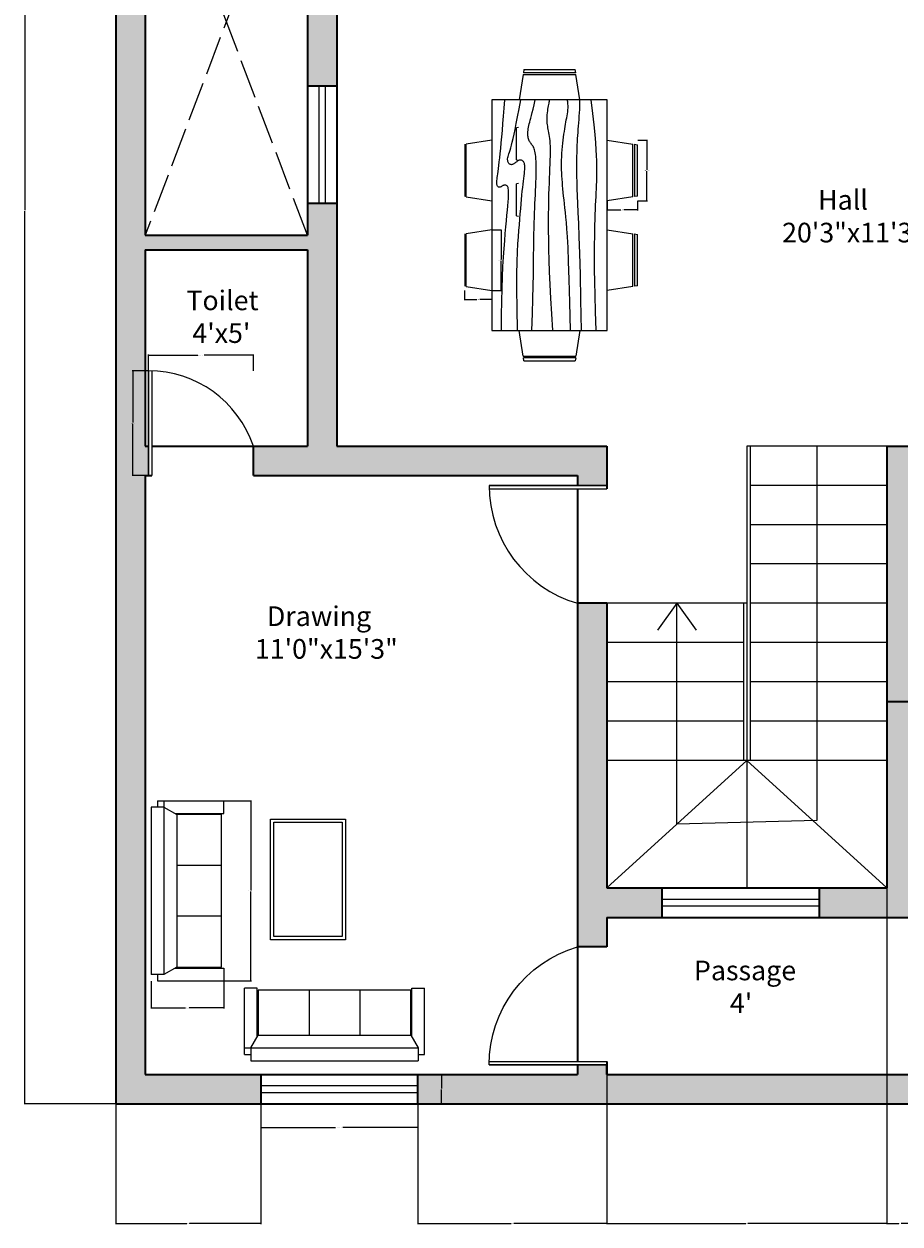
# Model space of a CAD drawing. Units: inches. Extents: x 1752 to 2227, y 6273 to 6884.
# Tile 1 of 6: x 1752 to 2020, y 6273 to 6640. Entities that reach past the tile are written whole.
import ezdxf

# ---------------------------------------------------------------- set-up
doc = ezdxf.new("R2010")
doc.units = ezdxf.units.IN
doc.header["$MEASUREMENT"] = 0
doc.linetypes.add('ACAD_ISO02W100', pattern=[15, 12, -3])
for name, color, linetype, lineweight in [('A-ANNO-DIMS', 2, 'Continuous', 18), ('A-AREA-IDEN', 7, 'Continuous', 18), ('A-DOOR', 3, 'Continuous', 20), ('A-FLOR-STRS', 7, 'Continuous', 20), ('A-FLOR-VOID', 8, 'ACAD_ISO02W100', 13), ('A-FURN', 8, 'Continuous', 18), ('A-GLAZ', 4, 'Continuous', 18), ('A-WALL', 7, 'Continuous', 35)]:
    doc.layers.add(name, color=color, linetype=linetype, lineweight=lineweight)
doc.layers.add('A-WALL-PATT', color=32, linetype='Continuous', lineweight=13, true_color=0xcd6928)
doc.styles.get("Standard").update_dxf_attribs({"font": 'arial.ttf'})
doc.dimstyles.get("Standard").update_dxf_attribs({"dimtxt": 0.18, "dimasz": 0.18, "dimexe": 0.18, "dimexo": 0.0625, "dimgap": 0.09, "dimtad": 0, "dimtih": 1, "dimtoh": 1, "dimdec": 4, "dimzin": 0, "dimdsep": 46, "dimtxsty": 'Standard', "dimcen": 0.09, "dimadec": 0, "dimazin": 0, "dimtfac": 1, "dimtdec": 4, "dimtofl": 0, "dimtmove": 0, "dimatfit": 3, "dimfxl": 1, "dimtolj": 1, "dimtzin": 0, "dimarcsym": 0})

# ---------------------------------------------------------------- blocks, each defined once
blk = doc.blocks.new('SOFA-TWO-SEAT')
for p, q in [((1.96, 55.04), (22.23, 55.04)), ((1.96, 55.04), (1.96, 53.08)), ((3.92, 55.04), (3.92, 1.96)), ((22.23, 51.12), (22.23, 55.04)), ((0, 53.08), (0, 1.96)), ((3.92, 53.08), (0, 53.08)), ((3.92, 53.08), (7.85, 50.88)), ((7.54, 51.12), (22.23, 51.12)), ((21.58, 50.87), (7.85, 50.87)), ((21.58, 35.3), (7.85, 35.3)), ((21.58, 19.74), (7.85, 19.74)), ((7.85, 4.17), (3.92, 1.96)), ((7.29, 3.92), (22.23, 3.92)), ((22.23, 3.92), (22.23, 0)), ((3.92, 1.96), (0, 1.96)), ((1.96, 1.96), (1.96, 0)), ((1.96, 0), (22.23, 0))]:
    blk.add_line(p, q)
blk.add_lwpolyline([(7.85, 50.88), (7.85, 4.17), (21.58, 4.17), (21.58, 50.87)])
blk = doc.blocks.new('CHAIR-DINING')
for p, q in [((0, 18.56), (7.83, 17.34)), ((7.83, 1.23), (7.83, 17.34)), ((8.32, 17.26), (8.32, 1.3)), ((8.32, 17.26), (9.3, 17.11)), ((9.3, 1.45), (9.3, 17.11)), ((7.83, 1.22), (0, 0)), ((9.3, 1.45), (8.32, 1.3))]:
    blk.add_line(p, q)
blk = doc.blocks.new('CHAIR-DINING-SIDE')
for p, q in [((8.32, 18.56), (0.49, 17.34)), ((0, 17.26), (0, 1.3)), ((0.49, 1.23), (0.49, 17.34)), ((0.49, 1.22), (8.32, 0))]:
    blk.add_line(p, q)
blk = doc.blocks.new('DOOR-SINGLE-36IN')
for p, q in [((35, 36), (35, 0)), ((36, 0), (36, 36)), ((36, 0), (35, 0))]:
    blk.add_line(p, q)
blk.add_arc((36, -1.5), 37.5, 90, 163.7398)
blk = doc.blocks.new('DOOR-SINGLE-32IN')
for p, q in [((32, 32), (31, 32)), ((31, 0), (31, 32)), ((32, 32), (32, 0))]:
    blk.add_line(p, q)
blk.add_arc((32, 33.76), 33.76, 198.5866, 270)
blk = doc.blocks.new('WINDOW-36IN')
for p, q in [((36, 9), (0, 9)), ((36, 5.5), (0, 5.5)), ((0, 3.5), (36, 3.5)), ((0, 0), (36, 0))]:
    blk.add_line(p, q)
blk = doc.blocks.new('WINDOW-48IN')
for p, q in [((48, 9), (0, 9)), ((48, 5.5), (0, 5.5)), ((0, 3.5), (48, 3.5)), ((0, 0), (48, 0))]:
    blk.add_line(p, q)
blk = doc.blocks.new('*D16')
at = {"layer": 'A-ANNO-DIMS', "color": 0, "lineweight": -2, "transparency": 16777216}
for p, q in [((1813.18, 6402.55), (1821.55, 6402.55)), ((1821.37, 6402.37), (1821.37, 6375.22)), ((1821.37, 6347.69), (1821.37, 6374.85)), ((1813.18, 6347.51), (1821.55, 6347.51))]:
    blk.add_line(p, q, dxfattribs=at)
at = {"layer": 'A-ANNO-DIMS', "color": 0, "transparency": 16777216}
for points in [[(1821.34, 6402.37), (1821.4, 6402.37), (1821.37, 6402.55)], [(1821.34, 6347.69), (1821.4, 6347.69), (1821.37, 6347.51)]]:
    blk.add_solid(points, dxfattribs=at)
at = {"layer": 'Defpoints', "color": 0, "transparency": 16777216}
for p in [(1813.11, 6402.55), (1821.37, 6402.55), (1813.11, 6347.51)]:
    blk.add_point(p, dxfattribs=at)
at = {"layer": 'A-ANNO-DIMS', "color": 0, "transparency": 16777216, "insert": (1821.37, 6375.03), "char_height": 0.18, "attachment_point": 5}
blk.add_mtext('\\A1;SOFA 55 TYP.', dxfattribs=at)
blk = doc.blocks.new('*D17')
at = {"layer": 'A-ANNO-DIMS', "color": 0, "lineweight": -2, "transparency": 16777216}
for p, q in [((1790.89, 6347.45), (1790.89, 6339.07)), ((1813.11, 6347.45), (1813.11, 6339.07)), ((1791.07, 6339.25), (1801.47, 6339.25)), ((1812.93, 6339.25), (1802.53, 6339.25))]:
    blk.add_line(p, q, dxfattribs=at)
at = {"layer": 'A-ANNO-DIMS', "color": 0, "transparency": 16777216}
for points in [[(1791.07, 6339.28), (1791.07, 6339.22), (1790.89, 6339.25)], [(1812.93, 6339.28), (1812.93, 6339.22), (1813.11, 6339.25)]]:
    blk.add_solid(points, dxfattribs=at)
at = {"layer": 'Defpoints', "color": 0, "transparency": 16777216}
for p in [(1790.89, 6347.51), (1813.11, 6347.51), (1813.11, 6339.25)]:
    blk.add_point(p, dxfattribs=at)
at = {"layer": 'A-ANNO-DIMS', "color": 0, "transparency": 16777216, "insert": (1802, 6339.25), "char_height": 0.18, "attachment_point": 5}
blk.add_mtext('\\A1;22 TYP.', dxfattribs=at)
blk = doc.blocks.new('*D20')
at = {"layer": 'A-ANNO-DIMS', "color": 0, "lineweight": -2, "transparency": 16777216}
for p, q in [((1790.15, 6533.98), (1790.15, 6538.89)), ((1790.33, 6538.71), (1805.21, 6538.71)), ((1821.97, 6538.71), (1807.08, 6538.71)), ((1822.15, 6533.98), (1822.15, 6538.89))]:
    blk.add_line(p, q, dxfattribs=at)
at = {"layer": 'A-ANNO-DIMS', "color": 0, "transparency": 16777216}
for points in [[(1790.33, 6538.74), (1790.33, 6538.68), (1790.15, 6538.71)], [(1821.97, 6538.74), (1821.97, 6538.68), (1822.15, 6538.71)]]:
    blk.add_solid(points, dxfattribs=at)
at = {"layer": 'Defpoints', "color": 0, "transparency": 16777216}
for p in [(1790.15, 6538.71), (1790.15, 6533.91), (1822.15, 6533.91)]:
    blk.add_point(p, dxfattribs=at)
at = {"layer": 'A-ANNO-DIMS', "color": 0, "transparency": 16777216, "insert": (1806.15, 6538.71), "char_height": 0.18, "attachment_point": 5}
blk.add_mtext('\\A1;DOOR 32 TYP.', dxfattribs=at)
blk = doc.blocks.new('*D21')
at = {"layer": 'A-ANNO-DIMS', "color": 0, "lineweight": -2, "transparency": 16777216}
for p, q in [((1790.08, 6533.91), (1785.17, 6533.91)), ((1785.35, 6533.73), (1785.35, 6518.1)), ((1785.35, 6502.09), (1785.35, 6517.73)), ((1790.08, 6501.91), (1785.17, 6501.91))]:
    blk.add_line(p, q, dxfattribs=at)
at = {"layer": 'A-ANNO-DIMS', "color": 0, "transparency": 16777216}
for points in [[(1785.32, 6533.73), (1785.38, 6533.73), (1785.35, 6533.91)], [(1785.32, 6502.09), (1785.38, 6502.09), (1785.35, 6501.91)]]:
    blk.add_solid(points, dxfattribs=at)
at = {"layer": 'Defpoints', "color": 0, "transparency": 16777216}
for p in [(1790.15, 6533.91), (1785.35, 6501.91), (1790.15, 6501.91)]:
    blk.add_point(p, dxfattribs=at)
at = {"layer": 'A-ANNO-DIMS', "color": 0, "transparency": 16777216, "insert": (1785.35, 6517.91), "char_height": 0.18, "attachment_point": 5}
blk.add_mtext('\\A1;32 TYP.', dxfattribs=at)
blk = doc.blocks.new('*D24')
at = {"layer": 'A-ANNO-DIMS', "color": 0, "lineweight": -2, "transparency": 16777216}
for p, q in [((1824.39, 6309.85), (1824.39, 6302.53)), ((1872.39, 6309.85), (1872.39, 6302.53)), ((1824.57, 6302.71), (1847.27, 6302.71)), ((1872.21, 6302.71), (1849.5, 6302.71))]:
    blk.add_line(p, q, dxfattribs=at)
at = {"layer": 'A-ANNO-DIMS', "color": 0, "transparency": 16777216}
for points in [[(1824.57, 6302.74), (1824.57, 6302.68), (1824.39, 6302.71)], [(1872.21, 6302.74), (1872.21, 6302.68), (1872.39, 6302.71)]]:
    blk.add_solid(points, dxfattribs=at)
at = {"layer": 'Defpoints', "color": 0, "transparency": 16777216}
for p in [(1824.39, 6309.91), (1872.39, 6309.91), (1824.39, 6302.71)]:
    blk.add_point(p, dxfattribs=at)
at = {"layer": 'A-ANNO-DIMS', "color": 0, "transparency": 16777216, "insert": (1848.39, 6302.71), "char_height": 0.18, "attachment_point": 5}
blk.add_mtext('\\A1;WINDOW 48 TYP.', dxfattribs=at)
blk = doc.blocks.new('*D25')
at = {"layer": 'A-ANNO-DIMS', "color": 0, "lineweight": -2, "transparency": 16777216}
for p, q in [((1872.45, 6318.91), (1879.77, 6318.91)), ((1879.59, 6318.73), (1879.59, 6314.6)), ((1879.59, 6310.09), (1879.59, 6314.23)), ((1872.45, 6309.91), (1879.77, 6309.91))]:
    blk.add_line(p, q, dxfattribs=at)
at = {"layer": 'A-ANNO-DIMS', "color": 0, "transparency": 16777216}
for points in [[(1879.56, 6318.73), (1879.62, 6318.73), (1879.59, 6318.91)], [(1879.56, 6310.09), (1879.62, 6310.09), (1879.59, 6309.91)]]:
    blk.add_solid(points, dxfattribs=at)
at = {"layer": 'Defpoints', "color": 0, "transparency": 16777216}
for p in [(1872.39, 6318.91), (1872.39, 6309.91), (1879.59, 6309.91)]:
    blk.add_point(p, dxfattribs=at)
at = {"layer": 'A-ANNO-DIMS', "color": 0, "transparency": 16777216, "insert": (1879.59, 6314.41), "char_height": 0.18, "attachment_point": 5}
blk.add_mtext('\\A1;9 TYP.', dxfattribs=at)
blk = doc.blocks.new('*D28')
at = {"layer": 'A-ANNO-DIMS', "color": 0, "lineweight": -2, "transparency": 16777216}
for p, q in [((1939.59, 6604.45), (1942.49, 6604.45)), ((1942.31, 6604.27), (1942.31, 6595.35)), ((1942.31, 6586.07), (1942.31, 6594.99)), ((1939.59, 6585.89), (1942.49, 6585.89))]:
    blk.add_line(p, q, dxfattribs=at)
at = {"layer": 'A-ANNO-DIMS', "color": 0, "transparency": 16777216}
for points in [[(1942.28, 6604.27), (1942.34, 6604.27), (1942.31, 6604.45)], [(1942.28, 6586.07), (1942.34, 6586.07), (1942.31, 6585.89)]]:
    blk.add_solid(points, dxfattribs=at)
at = {"layer": 'Defpoints', "color": 0, "transparency": 16777216}
for p in [(1939.53, 6604.45), (1942.31, 6604.45), (1939.53, 6585.89)]:
    blk.add_point(p, dxfattribs=at)
at = {"layer": 'A-ANNO-DIMS', "color": 0, "transparency": 16777216, "insert": (1942.31, 6595.17), "char_height": 0.18, "attachment_point": 5}
blk.add_mtext('\\A1;CHAIR A 19 TYP.', dxfattribs=at)
blk = doc.blocks.new('*D29')
at = {"layer": 'A-ANNO-DIMS', "color": 0, "lineweight": -2, "transparency": 16777216}
for p, q in [((1930.23, 6585.83), (1930.23, 6582.92)), ((1939.53, 6585.83), (1939.53, 6582.92)), ((1930.41, 6583.1), (1934.42, 6583.1)), ((1939.35, 6583.1), (1935.34, 6583.1))]:
    blk.add_line(p, q, dxfattribs=at)
at = {"layer": 'A-ANNO-DIMS', "color": 0, "transparency": 16777216}
for points in [[(1930.41, 6583.13), (1930.41, 6583.07), (1930.23, 6583.1)], [(1939.35, 6583.13), (1939.35, 6583.07), (1939.53, 6583.1)]]:
    blk.add_solid(points, dxfattribs=at)
at = {"layer": 'Defpoints', "color": 0, "transparency": 16777216}
for p in [(1930.23, 6585.89), (1939.53, 6585.89), (1939.53, 6583.1)]:
    blk.add_point(p, dxfattribs=at)
at = {"layer": 'A-ANNO-DIMS', "color": 0, "transparency": 16777216, "insert": (1934.88, 6583.1), "char_height": 0.18, "attachment_point": 5}
blk.add_mtext('\\A1;9 TYP.', dxfattribs=at)
blk = doc.blocks.new('*D30')
at = {"layer": 'A-ANNO-DIMS', "color": 0, "lineweight": -2, "transparency": 16777216}
for p, q in [((1895.08, 6577.05), (1897.98, 6577.05)), ((1897.8, 6576.87), (1897.8, 6567.96)), ((1897.8, 6558.67), (1897.8, 6567.59)), ((1895.08, 6558.49), (1897.98, 6558.49))]:
    blk.add_line(p, q, dxfattribs=at)
at = {"layer": 'A-ANNO-DIMS', "color": 0, "transparency": 16777216}
for points in [[(1897.77, 6576.87), (1897.83, 6576.87), (1897.8, 6577.05)], [(1897.77, 6558.67), (1897.83, 6558.67), (1897.8, 6558.49)]]:
    blk.add_solid(points, dxfattribs=at)
at = {"layer": 'Defpoints', "color": 0, "transparency": 16777216}
for p in [(1895.01, 6577.05), (1897.8, 6577.05), (1895.01, 6558.49)]:
    blk.add_point(p, dxfattribs=at)
at = {"layer": 'A-ANNO-DIMS', "color": 0, "transparency": 16777216, "insert": (1897.8, 6567.77), "char_height": 0.18, "attachment_point": 5}
blk.add_mtext('\\A1;CHAIR B 19 TYP.', dxfattribs=at)
blk = doc.blocks.new('*D31')
at = {"layer": 'A-ANNO-DIMS', "color": 0, "lineweight": -2, "transparency": 16777216}
for p, q in [((1886.69, 6558.43), (1886.69, 6555.53)), ((1895.01, 6558.43), (1895.01, 6555.53)), ((1886.87, 6555.71), (1890.4, 6555.71)), ((1894.83, 6555.71), (1891.31, 6555.71))]:
    blk.add_line(p, q, dxfattribs=at)
at = {"layer": 'A-ANNO-DIMS', "color": 0, "transparency": 16777216}
for points in [[(1886.87, 6555.74), (1886.87, 6555.68), (1886.69, 6555.71)], [(1894.83, 6555.74), (1894.83, 6555.68), (1895.01, 6555.71)]]:
    blk.add_solid(points, dxfattribs=at)
at = {"layer": 'Defpoints', "color": 0, "transparency": 16777216}
for p in [(1886.69, 6558.49), (1895.01, 6558.49), (1895.01, 6555.71)]:
    blk.add_point(p, dxfattribs=at)
at = {"layer": 'A-ANNO-DIMS', "color": 0, "transparency": 16777216, "insert": (1890.85, 6555.71), "char_height": 0.18, "attachment_point": 5}
blk.add_mtext('\\A1;8 TYP.', dxfattribs=at)
blk = doc.blocks.new('*D41')
at = {"layer": 'A-ANNO-DIMS', "color": 0, "lineweight": -2, "transparency": 16777216}
for p, q in [((1780.08, 6855.91), (1752.12, 6855.91)), ((1752.3, 6855.73), (1752.3, 6583.1)), ((1752.3, 6310.09), (1752.3, 6582.73)), ((1780.08, 6309.91), (1752.12, 6309.91))]:
    blk.add_line(p, q, dxfattribs=at)
at = {"layer": 'A-ANNO-DIMS', "color": 0, "transparency": 16777216}
for points in [[(1752.27, 6855.73), (1752.33, 6855.73), (1752.3, 6855.91)], [(1752.27, 6310.09), (1752.33, 6310.09), (1752.3, 6309.91)]]:
    blk.add_solid(points, dxfattribs=at)
at = {"layer": 'Defpoints', "color": 0, "transparency": 16777216}
for p in [(1752.3, 6855.91), (1780.15, 6855.91), (1780.15, 6309.91)]:
    blk.add_point(p, dxfattribs=at)
at = {"layer": 'A-ANNO-DIMS', "color": 0, "transparency": 16777216, "insert": (1752.3, 6582.91), "char_height": 0.18, "attachment_point": 5}
blk.add_mtext('\\A1;546', dxfattribs=at)
blk = doc.blocks.new('*D47')
at = {"layer": 'A-ANNO-DIMS', "color": 0, "lineweight": -2, "transparency": 16777216}
for p, q in [((1780.15, 6309.85), (1780.15, 6273.23)), ((1824.39, 6309.85), (1824.39, 6273.23)), ((1780.33, 6273.41), (1801.87, 6273.41)), ((1824.21, 6273.41), (1802.66, 6273.41))]:
    blk.add_line(p, q, dxfattribs=at)
at = {"layer": 'A-ANNO-DIMS', "color": 0, "transparency": 16777216}
for points in [[(1780.33, 6273.44), (1780.33, 6273.38), (1780.15, 6273.41)], [(1824.21, 6273.44), (1824.21, 6273.38), (1824.39, 6273.41)]]:
    blk.add_solid(points, dxfattribs=at)
at = {"layer": 'Defpoints', "color": 0, "transparency": 16777216}
for p in [(1780.15, 6309.91), (1824.39, 6309.91), (1824.39, 6273.41)]:
    blk.add_point(p, dxfattribs=at)
at = {"layer": 'A-ANNO-DIMS', "color": 0, "transparency": 16777216, "insert": (1802.27, 6273.41), "char_height": 0.18, "attachment_point": 5}
blk.add_mtext('\\A1;44.24', dxfattribs=at)
blk = doc.blocks.new('*D48')
at = {"layer": 'A-ANNO-DIMS', "color": 0, "lineweight": -2, "transparency": 16777216}
for p, q in [((1930.15, 6318.85), (1930.15, 6273.23)), ((1872.39, 6309.85), (1872.39, 6273.23)), ((1872.57, 6273.41), (1900.87, 6273.41)), ((1929.97, 6273.41), (1901.66, 6273.41))]:
    blk.add_line(p, q, dxfattribs=at)
at = {"layer": 'A-ANNO-DIMS', "color": 0, "transparency": 16777216}
for points in [[(1872.57, 6273.44), (1872.57, 6273.38), (1872.39, 6273.41)], [(1929.97, 6273.44), (1929.97, 6273.38), (1930.15, 6273.41)]]:
    blk.add_solid(points, dxfattribs=at)
at = {"layer": 'Defpoints', "color": 0, "transparency": 16777216}
for p in [(1930.15, 6318.91), (1872.39, 6309.91), (1930.15, 6273.41)]:
    blk.add_point(p, dxfattribs=at)
at = {"layer": 'A-ANNO-DIMS', "color": 0, "transparency": 16777216, "insert": (1901.27, 6273.41), "char_height": 0.18, "attachment_point": 5}
blk.add_mtext('\\A1;57.76', dxfattribs=at)
blk = doc.blocks.new('*D49')
at = {"layer": 'A-ANNO-DIMS', "color": 0, "lineweight": -2, "transparency": 16777216}
for p, q in [((2015.65, 6375.85), (2015.65, 6273.23)), ((1930.15, 6318.85), (1930.15, 6273.23)), ((1930.33, 6273.41), (1972.57, 6273.41)), ((2015.47, 6273.41), (1973.22, 6273.41))]:
    blk.add_line(p, q, dxfattribs=at)
at = {"layer": 'A-ANNO-DIMS', "color": 0, "transparency": 16777216}
for points in [[(1930.33, 6273.44), (1930.33, 6273.38), (1930.15, 6273.41)], [(2015.47, 6273.44), (2015.47, 6273.38), (2015.65, 6273.41)]]:
    blk.add_solid(points, dxfattribs=at)
at = {"layer": 'Defpoints', "color": 0, "transparency": 16777216}
for p in [(2015.65, 6375.91), (1930.15, 6318.91), (2015.65, 6273.41)]:
    blk.add_point(p, dxfattribs=at)
at = {"layer": 'A-ANNO-DIMS', "color": 0, "transparency": 16777216, "insert": (1972.9, 6273.41), "char_height": 0.18, "attachment_point": 5}
blk.add_mtext('\\A1;85.5', dxfattribs=at)
blk = doc.blocks.new('*D50')
at = {"layer": 'A-ANNO-DIMS', "color": 0, "lineweight": -2, "transparency": 16777216}
for p, q in [((2015.65, 6375.85), (2015.65, 6273.23)), ((2023.68, 6309.85), (2023.68, 6273.23)), ((2015.83, 6273.41), (2019.29, 6273.41)), ((2023.5, 6273.41), (2020.04, 6273.41))]:
    blk.add_line(p, q, dxfattribs=at)
at = {"layer": 'A-ANNO-DIMS', "color": 0, "transparency": 16777216}
for points in [[(2015.83, 6273.44), (2015.83, 6273.38), (2015.65, 6273.41)], [(2023.5, 6273.44), (2023.5, 6273.38), (2023.68, 6273.41)]]:
    blk.add_solid(points, dxfattribs=at)
at = {"layer": 'Defpoints', "color": 0, "transparency": 16777216}
for p in [(2015.65, 6375.91), (2023.68, 6309.91), (2023.68, 6273.41)]:
    blk.add_point(p, dxfattribs=at)
at = {"layer": 'A-ANNO-DIMS', "color": 0, "transparency": 16777216, "insert": (2019.66, 6273.41), "char_height": 0.18, "attachment_point": 5}
blk.add_mtext('\\A1;8.031', dxfattribs=at)

msp = doc.modelspace()

# ---------------------------------------------------------------- hatches: boundary and pattern name
at = {"layer": 'A-WALL-PATT'}
h = msp.add_hatch(color=256, dxfattribs=at)
h.dxf.hatch_style = 1
h.paths.add_polyline_path([(2198.6473, 6855.914), (1780.1473, 6855.914), (1780.1473, 6309.914), (1824.3861, 6309.914), (1824.3861, 6318.914), (1789.1473, 6318.914), (1789.1473, 6501.914), (1790.1473, 6501.914), (1790.1473, 6510.914), (1789.1473, 6510.914), (1789.1473, 6570.914), (1838.6473, 6570.914), (1838.6473, 6510.914), (1822.1473, 6510.914), (1822.1473, 6501.914), (1921.1473, 6501.914), (1921.1473, 6498.914), (1930.1473, 6498.914), (1930.1473, 6501.914), (1930.1473, 6510.914), (1847.6473, 6510.914), (1847.6473, 6585.039), (1838.6473, 6585.039), (1838.6473, 6575.414), (1789.1473, 6575.414), (1789.1473, 6705.914), (1795.2039, 6705.914), (1795.2039, 6714.914), (1789.1473, 6714.914), (1789.1473, 6846.914), (1984.1473, 6846.914), (1984.1473, 6714.914), (1977.8419, 6714.914), (1977.8419, 6705.914), (1984.1473, 6705.914), (1984.1473, 6651.914), (1977.6147, 6651.914), (1977.6147, 6642.914), (1996.1473, 6642.914), (1996.1473, 6651.914), (1993.1473, 6651.914), (1993.1473, 6846.914), (2125.1473, 6846.914), (2125.1473, 6840.4779), (2129.6473, 6840.4779), (2129.6473, 6846.914), (2189.6473, 6846.914), (2189.6473, 6798.914), (2162.6473, 6798.914), (2162.6473, 6794.414), (2189.6473, 6794.414), (2189.6473, 6710.414), (2175.6868, 6710.414), (2175.6868, 6705.914), (2189.6473, 6705.914), (2189.6473, 6651.914), (2164.6473, 6651.914), (2164.6473, 6642.914), (2189.6473, 6642.914), (2189.6473, 6510.914), (2166.7624, 6510.914), (2166.7624, 6501.914), (2189.6473, 6501.914), (2189.6473, 6318.914), (2173.9269, 6318.914), (2173.9269, 6309.914), (2198.6473, 6309.914)])
h.paths.add_polyline_path([(2023.6785, 6318.914), (1930.1473, 6318.914), (1930.1473, 6321.914), (1921.1473, 6321.914), (1921.1473, 6318.914), (1872.3861, 6318.914), (1872.3861, 6309.914), (2023.6785, 6309.914)], flags=17)
h.paths.add_polyline_path([(2092.7496, 6318.914), (2061.7431, 6318.914), (2061.7431, 6309.914), (2092.7496, 6309.914)], flags=0)
h.paths.add_polyline_path([(1947.0033, 6375.914), (1930.1473, 6375.914), (1930.1473, 6462.914), (1921.1473, 6462.914), (1921.1473, 6357.914), (1930.1473, 6357.914), (1930.1473, 6366.914), (1947.0033, 6366.914)], flags=17)
h.paths.add_polyline_path([(2024.6473, 6432.914), (2015.6473, 6432.914), (2015.6473, 6375.914), (1995.0033, 6375.914), (1995.0033, 6366.914), (2024.6473, 6366.914)], flags=17)
h.paths.add_polyline_path([(2030.6473, 6441.914), (2024.6473, 6441.914), (2024.6473, 6510.914), (2015.6473, 6510.914), (2015.6473, 6432.914), (2024.6473, 6432.914), (2030.6473, 6432.914)], flags=17)
h.paths.add_polyline_path([(2093.6473, 6501.914), (2118.7624, 6501.914), (2118.7624, 6510.914), (2093.6473, 6510.914), (2093.6473, 6603.914), (2084.6473, 6603.914), (2084.6473, 6441.914), (2078.6473, 6441.914), (2078.6473, 6432.914), (2093.6473, 6432.914)], flags=17)
h.paths.add_polyline_path([(2132.6473, 6651.914), (2129.6473, 6651.914), (2129.6473, 6705.914), (2139.6868, 6705.914), (2139.6868, 6710.414), (2129.6473, 6710.414), (2129.6473, 6794.414), (2130.6473, 6794.414), (2130.6473, 6798.914), (2129.6473, 6798.914), (2129.6473, 6804.4779), (2125.1473, 6804.4779), (2125.1473, 6651.914), (2032.1473, 6651.914), (2032.1473, 6642.914), (2084.6473, 6642.914), (2084.6473, 6639.914), (2093.6473, 6639.914), (2093.6473, 6642.914), (2132.6473, 6642.914)], flags=17)
h.paths.add_polyline_path([(1929.6147, 6651.914), (1924.1473, 6651.914), (1924.1473, 6705.914), (1941.8419, 6705.914), (1941.8419, 6714.914), (1911.8299, 6714.914), (1911.8299, 6705.914), (1919.6473, 6705.914), (1919.6473, 6651.914), (1847.6473, 6651.914), (1847.6473, 6662.4635), (1838.6473, 6662.4635), (1838.6473, 6621.039), (1847.6473, 6621.039), (1847.6473, 6642.914), (1929.6147, 6642.914)], flags=17)
h.paths.add_polyline_path([(1879.8299, 6714.914), (1831.2039, 6714.914), (1831.2039, 6705.914), (1838.6473, 6705.914), (1838.6473, 6698.4635), (1847.6473, 6698.4635), (1847.6473, 6705.914), (1879.8299, 6705.914)], flags=17)

# ---------------------------------------------------------------- linework, layer by layer
at = {"layer": 'A-DOOR'}
for p, q in [((1790.1473, 6533.914), (1790.1473, 6501.914)), ((1894.1473, 6498.914), (1930.1473, 6498.914)), ((1894.1473, 6321.914), (1930.1473, 6321.914))]:
    msp.add_line(p, q, dxfattribs=at)
at = {"layer": 'A-FLOR-STRS'}
for p, q in [((2015.6473, 6510.914), (1972.8973, 6510.914)), ((1972.8973, 6510.914), (1972.8973, 6414.914)), ((1973.8973, 6510.914), (1973.8973, 6414.914)), ((1994.2723, 6510.914), (1994.2723, 6396.5166)), ((2015.6473, 6498.914), (1973.8973, 6498.914)), ((2015.6473, 6486.914), (1973.8973, 6486.914)), ((2015.6473, 6474.914), (1973.8973, 6474.914)), ((1972.8973, 6462.914), (1930.1473, 6462.914)), ((1951.5223, 6462.914), (1945.6334, 6454.6748)), ((1951.5223, 6395.414), (1951.5223, 6462.914)), ((1951.5223, 6462.914), (1957.4112, 6454.6748)), ((1971.8973, 6462.914), (1971.8973, 6414.914)), ((2015.6473, 6462.914), (1973.8973, 6462.914)), ((1971.8973, 6450.914), (1930.1473, 6450.914)), ((2015.6473, 6450.914), (1973.8973, 6450.914)), ((1971.8973, 6438.914), (1930.1473, 6438.914)), ((2015.6473, 6438.914), (1973.8973, 6438.914)), ((1971.8973, 6426.914), (1930.1473, 6426.914)), ((2015.6473, 6426.914), (1973.8973, 6426.914)), ((2015.6473, 6414.914), (1930.1473, 6414.914)), ((1972.8973, 6414.914), (1930.1473, 6375.914)), ((1972.8973, 6414.914), (1972.8973, 6375.914)), ((1972.8973, 6414.914), (2015.6473, 6375.914)), ((2015.6473, 6375.914), (2015.6473, 6414.914)), ((1994.2723, 6396.5166), (1951.5223, 6395.414))]:
    msp.add_line(p, q, dxfattribs=at)
at = {"layer": 'A-FLOR-VOID'}
for p, q in [((1838.6473, 6705.914), (1789.1473, 6575.414)), ((1838.6473, 6575.414), (1789.1473, 6705.914))]:
    msp.add_line(p, q, dxfattribs=at)
at = {"layer": 'A-FURN'}
for p, q in [((1904.7953, 6625.9895), (1904.6424, 6625.0115)), ((1904.7953, 6625.9895), (1920.4502, 6625.9895)), ((1920.6031, 6625.0107), (1920.4502, 6625.9895)), ((1904.566, 6624.5224), (1903.3425, 6616.692)), ((1904.5698, 6624.5218), (1920.6842, 6624.5218)), ((1920.6052, 6625.011), (1904.6452, 6625.011)), ((1921.9029, 6616.692), (1920.6796, 6624.5211)), ((1895.0109, 6616.6943), (1895.0109, 6546.2471)), ((1930.2345, 6616.6943), (1895.0109, 6616.6943)), ((1930.2345, 6546.2471), (1930.2345, 6616.6943)), ((1903.0909, 6608.2501), (1902.4808, 6608.1547)), ((1902.4808, 6598.3952), (1902.4808, 6608.1547)), ((1902.4808, 6598.3952), (1903.0905, 6598.2999)), ((1903.0909, 6591.1708), (1902.4808, 6591.0755)), ((1902.4808, 6581.3159), (1902.4808, 6591.0755)), ((1902.4808, 6581.3159), (1903.0905, 6581.2207)), ((1895.0109, 6546.2471), (1930.2345, 6546.2471)), ((1904.566, 6538.4191), (1903.3425, 6546.2495)), ((1921.9029, 6546.2495), (1920.6796, 6538.4204)), ((1904.5698, 6538.4197), (1920.6842, 6538.4197)), ((1904.7953, 6536.952), (1904.6424, 6537.9301)), ((1920.6052, 6537.9305), (1904.6452, 6537.9305)), ((1920.6031, 6537.9308), (1920.4502, 6536.952)), ((1904.7953, 6536.952), (1920.4502, 6536.952))]:
    msp.add_line(p, q, dxfattribs=at)
for points in [[(1897.9462, 6546.2471), (1897.9682, 6550.9659), (1898.0303, 6555.241), (1898.1268, 6559.1098), (1898.252, 6562.6105), (1898.4001, 6565.7804), (1898.5654, 6568.6575), (1898.7422, 6571.2795), (1898.9247, 6573.6841), (1899.1075, 6575.9031), (1899.2865, 6577.945), (1899.4578, 6579.8119), (1899.6177, 6581.5065), (1899.7623, 6583.0309), (1899.8878, 6584.3876), (1899.9904, 6585.579), (1900.0662, 6586.6075), (1900.1123, 6587.4776), (1900.1299, 6588.2026), (1900.1206, 6588.7975), (1900.0865, 6589.2779), (1900.0295, 6589.6588), (1899.9515, 6589.9556), (1899.8544, 6590.1836), (1899.74, 6590.3581), (1899.6105, 6590.4924), (1899.4686, 6590.5913), (1899.3172, 6590.6577), (1899.1591, 6590.6945), (1898.9971, 6590.7045), (1898.8342, 6590.6907), (1898.6732, 6590.6558), (1898.517, 6590.6028), (1898.3678, 6590.5348), (1898.2252, 6590.4563), (1898.0884, 6590.372), (1897.9564, 6590.2868), (1897.8282, 6590.2054), (1897.7029, 6590.1327), (1897.5795, 6590.0733), (1897.457, 6590.032), (1897.335, 6590.013), (1897.2149, 6590.0168), (1897.0987, 6590.0435), (1896.9882, 6590.0932), (1896.8853, 6590.1658), (1896.792, 6590.2614), (1896.7101, 6590.3799), (1896.6416, 6590.5213), (1896.5881, 6590.6865), (1896.5499, 6590.8805), (1896.527, 6591.1089), (1896.5193, 6591.3774), (1896.527, 6591.6918), (1896.5499, 6592.0577), (1896.5881, 6592.481), (1896.6416, 6592.9673), (1896.7103, 6593.5235), (1896.7933, 6594.1604), (1896.8896, 6594.8901), (1896.9984, 6595.7243), (1897.1186, 6596.6751), (1897.2493, 6597.7544), (1897.3896, 6598.9742), (1897.5385, 6600.3464), (1897.6951, 6601.8799), (1897.8583, 6603.5715), (1898.0273, 6605.4151), (1898.201, 6607.4043), (1898.3786, 6609.5331), (1898.559, 6611.7952), (1898.7414, 6614.1844), (1898.9247, 6616.6943)], [(1902.8384, 6546.2471), (1902.6987, 6553.1191), (1902.6384, 6558.798), (1902.6449, 6563.444), (1902.7059, 6567.2172), (1902.8089, 6570.2776), (1902.9416, 6572.7852), (1903.0914, 6574.9002), (1903.2461, 6576.7824), (1903.3953, 6578.565), (1903.5378, 6580.2726), (1903.6746, 6581.9027), (1903.8066, 6583.4531), (1903.9348, 6584.9213), (1904.0602, 6586.305), (1904.1836, 6587.6016), (1904.306, 6588.809), (1904.4279, 6589.9255), (1904.5468, 6590.9531), (1904.6601, 6591.8948), (1904.7647, 6592.7533), (1904.8578, 6593.5316), (1904.9367, 6594.2324), (1904.9983, 6594.8587), (1905.0399, 6595.4134), (1905.0591, 6595.8998), (1905.0564, 6596.3231), (1905.0327, 6596.689), (1904.9889, 6597.0034), (1904.926, 6597.2719), (1904.8449, 6597.5002), (1904.7467, 6597.6942), (1904.6322, 6597.8595), (1904.5026, 6598.0008), (1904.3595, 6598.1181), (1904.2051, 6598.2107), (1904.041, 6598.2774), (1903.8694, 6598.3174), (1903.692, 6598.3296), (1903.5107, 6598.3132), (1903.3276, 6598.2672), (1903.1441, 6598.1917), (1902.9607, 6598.0914), (1902.7772, 6597.9719), (1902.5938, 6597.8392), (1902.4103, 6597.6986), (1902.2269, 6597.5563), (1902.0434, 6597.4177), (1901.86, 6597.2888), (1901.6767, 6597.1746), (1901.4943, 6597.0785), (1901.3139, 6597.0036), (1901.1363, 6596.9524), (1900.9626, 6596.928), (1900.7936, 6596.9333), (1900.6304, 6596.9711), (1900.4738, 6597.0442), (1900.3254, 6597.1545), (1900.1885, 6597.3002), (1900.0668, 6597.4784), (1899.9642, 6597.6862), (1899.8846, 6597.9208), (1899.8317, 6598.1793), (1899.8094, 6598.4588), (1899.8216, 6598.7564), (1899.8707, 6599.0722), (1899.9547, 6599.417), (1900.0702, 6599.8048), (1900.2139, 6600.2495), (1900.3825, 6600.765), (1900.5726, 6601.3649), (1900.7808, 6602.0633), (1901.0038, 6602.874), (1901.2401, 6603.814), (1901.495, 6604.913), (1901.7756, 6606.2042), (1902.0893, 6607.7203), (1902.443, 6609.4944), (1902.8441, 6611.5595), (1903.2997, 6613.9485), (1903.8168, 6616.6943)], [(1907.2413, 6546.2471), (1907.403, 6551.4175), (1907.5254, 6555.964), (1907.6154, 6559.9505), (1907.6796, 6563.4411), (1907.7247, 6566.4998), (1907.7573, 6569.1906), (1907.7842, 6571.5776), (1907.8121, 6573.7248), (1907.8463, 6575.6892), (1907.8873, 6577.4997), (1907.9339, 6579.1784), (1907.9854, 6580.7471), (1908.0406, 6582.228), (1908.0987, 6583.6429), (1908.1588, 6585.0139), (1908.2198, 6586.3629), (1908.2806, 6587.7063), (1908.3395, 6589.0383), (1908.3946, 6590.3474), (1908.444, 6591.622), (1908.4857, 6592.8508), (1908.5179, 6594.0222), (1908.5386, 6595.1249), (1908.5459, 6596.1472), (1908.5383, 6597.0807), (1908.5153, 6597.927), (1908.4771, 6598.6913), (1908.4236, 6599.3781), (1908.3548, 6599.9924), (1908.2707, 6600.5387), (1908.1714, 6601.0221), (1908.0567, 6601.4471), (1907.9272, 6601.8191), (1907.7853, 6602.1452), (1907.6339, 6602.4332), (1907.4758, 6602.6905), (1907.3138, 6602.9249), (1907.1509, 6603.1441), (1906.9899, 6603.3556), (1906.8337, 6603.5671), (1906.6849, 6603.7854), (1906.5457, 6604.0142), (1906.418, 6604.2564), (1906.3037, 6604.5149), (1906.2046, 6604.7925), (1906.1228, 6605.0921), (1906.06, 6605.4164), (1906.0183, 6605.7686), (1905.999, 6606.1503), (1906.0017, 6606.5597), (1906.0255, 6606.994), (1906.0693, 6607.4502), (1906.1322, 6607.9255), (1906.2132, 6608.4172), (1906.3115, 6608.9222), (1906.426, 6609.4377), (1906.5566, 6609.9668), (1906.7063, 6610.5372), (1906.8789, 6611.1819), (1907.0783, 6611.9347), (1907.3082, 6612.8288), (1907.5726, 6613.898), (1907.8752, 6615.1753), (1908.2198, 6616.6943)], [(1913.6011, 6546.2471), (1913.2676, 6551.3433), (1912.9966, 6556.0124), (1912.782, 6560.2858), (1912.6176, 6564.1952), (1912.4972, 6567.7722), (1912.4144, 6571.0482), (1912.3632, 6574.0546), (1912.3373, 6576.8232), (1912.3312, 6579.3828), (1912.3418, 6581.7523), (1912.3667, 6583.9478), (1912.4036, 6585.9858), (1912.45, 6587.8823), (1912.5036, 6589.6537), (1912.562, 6591.316), (1912.6227, 6592.8858), (1912.6834, 6594.3762), (1912.7412, 6595.7892), (1912.7933, 6597.1239), (1912.8367, 6598.3793), (1912.8688, 6599.5544), (1912.8864, 6600.6483), (1912.8869, 6601.66), (1912.8673, 6602.5887), (1912.8259, 6603.4347), (1912.7654, 6604.2053), (1912.6896, 6604.909), (1912.6023, 6605.5545), (1912.5074, 6606.1503), (1912.4087, 6606.7049), (1912.3099, 6607.2271), (1912.215, 6607.7254), (1912.1275, 6608.2079), (1912.0494, 6608.6809), (1911.9828, 6609.15), (1911.9297, 6609.6211), (1911.8918, 6610.0998), (1911.8711, 6610.5919), (1911.8695, 6611.1031), (1911.8889, 6611.6392), (1911.9301, 6612.2022), (1911.9895, 6612.78), (1912.0623, 6613.3569), (1912.1437, 6613.9171), (1912.2289, 6614.4447), (1912.3131, 6614.9242), (1912.3916, 6615.3395), (1912.4597, 6615.6752), (1912.5135, 6615.9213), (1912.5539, 6616.0924), (1912.5829, 6616.209), (1912.6023, 6616.2918), (1912.6141, 6616.3611), (1912.6202, 6616.4377), (1912.6224, 6616.5419), (1912.6227, 6616.6943)], [(1918.9825, 6546.2471), (1918.7992, 6554.8727), (1918.6169, 6561.8199), (1918.4365, 6567.3138), (1918.2589, 6571.5794), (1918.0852, 6574.8417), (1917.9162, 6577.3258), (1917.753, 6579.2566), (1917.5964, 6580.8592), (1917.4474, 6582.3228), (1917.3059, 6583.6933), (1917.1722, 6584.9806), (1917.0461, 6586.1947), (1916.9276, 6587.3458), (1916.8167, 6588.444), (1916.7135, 6589.4991), (1916.618, 6590.5213), (1916.5304, 6591.5197), (1916.4524, 6592.501), (1916.3858, 6593.4709), (1916.3326, 6594.435), (1916.2947, 6595.3991), (1916.274, 6596.369), (1916.2724, 6597.3502), (1916.2918, 6598.3487), (1916.3334, 6599.3675), (1916.395, 6600.3986), (1916.4739, 6601.4317), (1916.567, 6602.4561), (1916.6717, 6603.4614), (1916.7849, 6604.4372), (1916.9038, 6605.3728), (1917.0257, 6606.2578), (1917.1479, 6607.0847), (1917.2696, 6607.8585), (1917.3904, 6608.5875), (1917.5098, 6609.2797), (1917.6272, 6609.9432), (1917.7423, 6610.5862), (1917.8545, 6611.2167), (1917.9633, 6611.843), (1918.0671, 6612.4711), (1918.1589, 6613.0998), (1918.2306, 6613.7256), (1918.2742, 6614.3451), (1918.2814, 6614.9551), (1918.2443, 6615.5522), (1918.1545, 6616.1331), (1918.0041, 6616.6943)], [(1922.407, 6546.2471), (1922.2241, 6555.638), (1922.044, 6563.4015), (1921.8696, 6569.7453), (1921.7038, 6574.8765), (1921.5495, 6579.0025), (1921.4095, 6582.3307), (1921.2867, 6585.0683), (1921.184, 6587.4228), (1921.1034, 6589.5689), (1921.0439, 6591.5507), (1921.0034, 6593.3795), (1920.9802, 6595.0669), (1920.9722, 6596.6243), (1920.9776, 6598.0633), (1920.9945, 6599.3953), (1921.0209, 6600.6318), (1921.0553, 6601.7846), (1921.0967, 6602.8676), (1921.1449, 6603.8953), (1921.1993, 6604.8818), (1921.2594, 6605.8417), (1921.3248, 6606.789), (1921.3949, 6607.7383), (1921.4694, 6608.7039), (1921.5472, 6609.696), (1921.6254, 6610.7091), (1921.7009, 6611.7337), (1921.77, 6612.7603), (1921.8297, 6613.7791), (1921.8764, 6614.7808), (1921.9069, 6615.7557), (1921.9178, 6616.6943)], [(1926.81, 6546.2471), (1926.6487, 6552.0315), (1926.5284, 6556.9774), (1926.4445, 6561.1867), (1926.3921, 6564.761), (1926.3665, 6567.802), (1926.3628, 6570.4118), (1926.3764, 6572.6919), (1926.4023, 6574.744), (1926.4366, 6576.6545), (1926.4775, 6578.4469), (1926.5241, 6580.1294), (1926.5756, 6581.7103), (1926.6308, 6583.1974), (1926.689, 6584.5991), (1926.749, 6585.9233), (1926.81, 6587.1782), (1926.8708, 6588.374), (1926.9291, 6589.5281), (1926.9827, 6590.6604), (1927.0291, 6591.7902), (1927.066, 6592.9372), (1927.0909, 6594.1209), (1927.1015, 6595.3611), (1927.0954, 6596.6773), (1927.0685, 6598.0976), (1927.0107, 6599.6845), (1926.9098, 6601.5094), (1926.7539, 6603.6435), (1926.5312, 6606.1578), (1926.2297, 6609.1236), (1925.8374, 6612.612), (1925.3423, 6616.6943)]]:
    msp.add_lwpolyline(points, dxfattribs=at)
for points in [[(1827.4238, 6396.9786), (1850.2891, 6396.9786), (1850.2891, 6360.035), (1827.4238, 6360.035)], [(1828.4238, 6395.9786), (1849.2891, 6395.9786), (1849.2891, 6361.035), (1828.4238, 6361.035)]]:
    msp.add_lwpolyline(points, close=True, dxfattribs=at)
at = {"layer": 'A-WALL'}
for p, q in [((1780.1473, 6855.914), (1780.1473, 6309.914)), ((1789.1473, 6705.914), (1789.1473, 6575.414)), ((1838.6473, 6705.914), (1838.6473, 6575.414)), ((1847.6473, 6642.914), (1847.6473, 6510.914)), ((1838.6473, 6621.039), (1847.6473, 6621.039)), ((1847.6473, 6585.039), (1838.6473, 6585.039)), ((1789.1473, 6575.414), (1838.6473, 6575.414)), ((1789.1473, 6570.914), (1838.6473, 6570.914)), ((1789.1473, 6570.914), (1789.1473, 6510.914)), ((1838.6473, 6570.914), (1838.6473, 6510.914)), ((1789.1473, 6510.914), (1790.1473, 6510.914)), ((1791.1473, 6510.914), (1838.6473, 6510.914)), ((1822.1473, 6501.914), (1822.1473, 6510.914)), ((1847.6473, 6510.914), (1930.1473, 6510.914)), ((1930.1473, 6510.914), (1930.1473, 6497.914)), ((2015.6473, 6510.914), (2015.6473, 6375.914)), ((2015.6473, 6510.914), (2024.6473, 6510.914)), ((1789.1473, 6501.914), (1791.1473, 6501.914)), ((1789.1473, 6501.914), (1790.1473, 6501.914)), ((1789.1473, 6501.914), (1789.1473, 6318.914)), ((1822.1473, 6501.914), (1921.1473, 6501.914)), ((1921.1473, 6501.914), (1921.1473, 6498.914)), ((1930.1473, 6501.914), (1930.1473, 6498.914)), ((1921.1473, 6497.914), (1921.1473, 6322.914)), ((1930.1473, 6462.914), (1921.1473, 6462.914)), ((1930.1473, 6462.914), (1930.1473, 6375.914)), ((2015.6473, 6432.914), (2093.6473, 6432.914)), ((1930.1473, 6375.914), (2015.6473, 6375.914)), ((1947.0033, 6366.914), (1947.0033, 6375.914)), ((1995.0033, 6375.914), (1995.0033, 6366.914)), ((1930.1473, 6366.914), (2024.6473, 6366.914)), ((1930.1473, 6366.914), (1930.1473, 6357.914)), ((1930.1473, 6357.914), (1921.1473, 6357.914)), ((1921.1473, 6321.914), (1921.1473, 6318.914)), ((1930.1473, 6322.914), (1930.1473, 6318.914)), ((1930.1473, 6318.914), (1930.1473, 6321.914)), ((1789.1473, 6318.914), (1921.1473, 6318.914)), ((1824.3861, 6318.914), (1824.3861, 6309.914)), ((1872.3861, 6309.914), (1872.3861, 6318.914)), ((1930.1473, 6318.914), (2023.6785, 6318.914)), ((1780.1473, 6309.914), (2023.6785, 6309.914))]:
    msp.add_line(p, q, dxfattribs=at)

# ---------------------------------------------------------------- block references
at = {"layer": 'A-DOOR'}
for name, p, rotation in [('DOOR-SINGLE-32IN', (1822.1472, 6533.9141), 180), ('DOOR-SINGLE-36IN', (1930.1473, 6462.9141), 90.00000000000412)]:
    msp.add_blockref(name, p, dxfattribs=dict(at, rotation=rotation))
at = {"layer": 'A-DOOR', "extrusion": (0, 0, -1), "zscale": -1, "rotation": 270.0000000000047}
msp.add_blockref('DOOR-SINGLE-36IN', (-1930.1473, 6357.9139), dxfattribs=at)
at = {"layer": 'A-FURN'}
for name, p in [('CHAIR-DINING-SIDE', (1886.694, 6585.889)), ('CHAIR-DINING', (1930.232, 6585.8891)), ('CHAIR-DINING-SIDE', (1886.694, 6558.4929)), ('CHAIR-DINING', (1930.232, 6558.493)), ('SOFA-TWO-SEAT', (1790.885, 6347.51))]:
    msp.add_blockref(name, p, dxfattribs=at)
at = {"layer": 'A-FURN', "rotation": 90.00000000000603}
msp.add_blockref('SOFA-TWO-SEAT', (1874.4517, 6323.1036), dxfattribs=at)
at = {"layer": 'A-GLAZ'}
for name, p, rotation in [('WINDOW-36IN', (1847.6473, 6585.0392), 90.00000000000954), ('WINDOW-48IN', (1995.0037, 6375.9141), 180), ('WINDOW-48IN', (1872.3865, 6318.9141), 180)]:
    msp.add_blockref(name, p, dxfattribs=dict(at, rotation=rotation))

# ---------------------------------------------------------------- texts
at = {"layer": 'A-AREA-IDEN', "char_height": 6, "attachment_point": 1}
for s, width, insert in [('      Hall\\P20\'3"x11\'3"', 75.076462, (1983.6553, 6589.178)), ("Toilet\\P 4'x5'", 34.504486, (1801.6889, 6558.4641)), ('  Drawing\\P11\'0"x15\'3"', 54.76029, (1822.6171, 6461.9632)), ("Passage\\P      4'", 53.315886, (1956.7218, 6353.7109))]:
    msp.add_mtext_dynamic_manual_height_columns(s, width=width, gutter_width=30, heights=[0], dxfattribs=dict(at, insert=insert))

# ---------------------------------------------------------------- dimensions: what is measured, and where the dimension line sits
at = {"layer": 'A-ANNO-DIMS'}
dim = msp.add_linear_dim(base=(1752.2973, 6855.914), p1=(1780.1473, 6309.914), p2=(1780.1473, 6855.914), angle=90, dimstyle='Standard', override={"dimdec": 0, "dimlfac": 1, "dimrnd": 0, "dimzin": 0, "dimdsep": 46, "dimlunit": 2}, dxfattribs=at)
dim.commit()
dim.dimension.update_dxf_attribs({"geometry": '*D41', "text_midpoint": (1752.2973, 6582.914)})
for base, p1, p2, angle, text, picture, middle in [((1942.3137, 6604.4491), (1939.5296, 6585.8887), (1939.5296, 6604.4491), 90, 'CHAIR A <> TYP.', '*D28', (1942.3137, 6595.1689)), ((1897.7973, 6577.0529), (1895.0132, 6558.4925), (1895.0132, 6577.0529), 90, 'CHAIR B <> TYP.', '*D30', (1897.7973, 6567.7727)), ((1790.1473, 6538.714), (1822.1473, 6533.914), (1790.1473, 6533.914), 180, 'DOOR <> TYP.', '*D20', (1806.1473, 6538.714)), ((1785.3473, 6501.914), (1790.1473, 6533.914), (1790.1473, 6501.914), 270, '<> TYP.', '*D21', (1785.3473, 6517.914)), ((1821.3709, 6402.554), (1813.1143, 6347.51), (1813.1143, 6402.554), 90, 'SOFA <> TYP.', '*D16', (1821.3709, 6375.032)), ((1879.5861, 6309.914), (1872.3861, 6318.914), (1872.3861, 6309.914), 270, '<> TYP.', '*D25', (1879.5861, 6314.414)), ((1824.3861, 6302.714), (1872.3861, 6309.914), (1824.3861, 6309.914), 180, 'WINDOW <> TYP.', '*D24', (1848.3861, 6302.714))]:
    dim = msp.add_linear_dim(base=base, p1=p1, p2=p2, angle=angle, text=text, dimstyle='Standard', override={"dimdec": 0, "dimlfac": 1, "dimrnd": 0, "dimzin": 0, "dimdsep": 46, "dimlunit": 2}, dxfattribs=at)
    dim.commit()
    dim.dimension.update_dxf_attribs({"geometry": picture, "text_midpoint": middle})
for base, p1, p2, picture, middle in [((1939.5296, 6583.1046), (1930.2322, 6585.8887), (1939.5296, 6585.8887), '*D29', (1934.8809, 6583.1046)), ((1895.0132, 6555.7085), (1886.6942, 6558.4925), (1895.0132, 6558.4925), '*D31', (1890.8537, 6555.7085)), ((1813.1143, 6339.2534), (1790.8853, 6347.51), (1813.1143, 6347.51), '*D17', (1801.9998, 6339.2534))]:
    dim = msp.add_linear_dim(base=base, p1=p1, p2=p2, text='<> TYP.', dimstyle='Standard', override={"dimdec": 0, "dimlfac": 1, "dimrnd": 0, "dimzin": 0, "dimdsep": 46, "dimlunit": 2}, dxfattribs=at)
    dim.commit()
    dim.dimension.update_dxf_attribs({"geometry": picture, "text_midpoint": middle})
for base, p1, p2, override, picture, middle in [((2015.6473, 6273.4139), (1930.1473, 6318.914), (2015.6473, 6375.914), {"dimdec": 1, "dimlfac": 1, "dimrnd": 0, "dimzin": 0, "dimdsep": 46, "dimlunit": 2}, '*D49', (1972.8973, 6273.4139)), ((2023.6785, 6273.4139), (2015.6473, 6375.914), (2023.6785, 6309.914), {"dimdec": 3, "dimlfac": 1, "dimrnd": 0, "dimzin": 0, "dimdsep": 46, "dimlunit": 2}, '*D50', (2019.6629, 6273.4139)), ((1930.1473, 6273.4139), (1872.3861, 6309.914), (1930.1473, 6318.914), {"dimdec": 2, "dimlfac": 1, "dimrnd": 0, "dimzin": 0, "dimdsep": 46, "dimlunit": 2}, '*D48', (1901.2667, 6273.4139)), ((1824.3861, 6273.4139), (1780.1473, 6309.914), (1824.3861, 6309.914), {"dimdec": 2, "dimlfac": 1, "dimrnd": 0, "dimzin": 0, "dimdsep": 46, "dimlunit": 2}, '*D47', (1802.2667, 6273.4139))]:
    dim = msp.add_linear_dim(base=base, p1=p1, p2=p2, dimstyle='Standard', override=override, dxfattribs=at)
    dim.commit()
    dim.dimension.update_dxf_attribs({"geometry": picture, "text_midpoint": middle})

doc.saveas('drawing.dxf')
